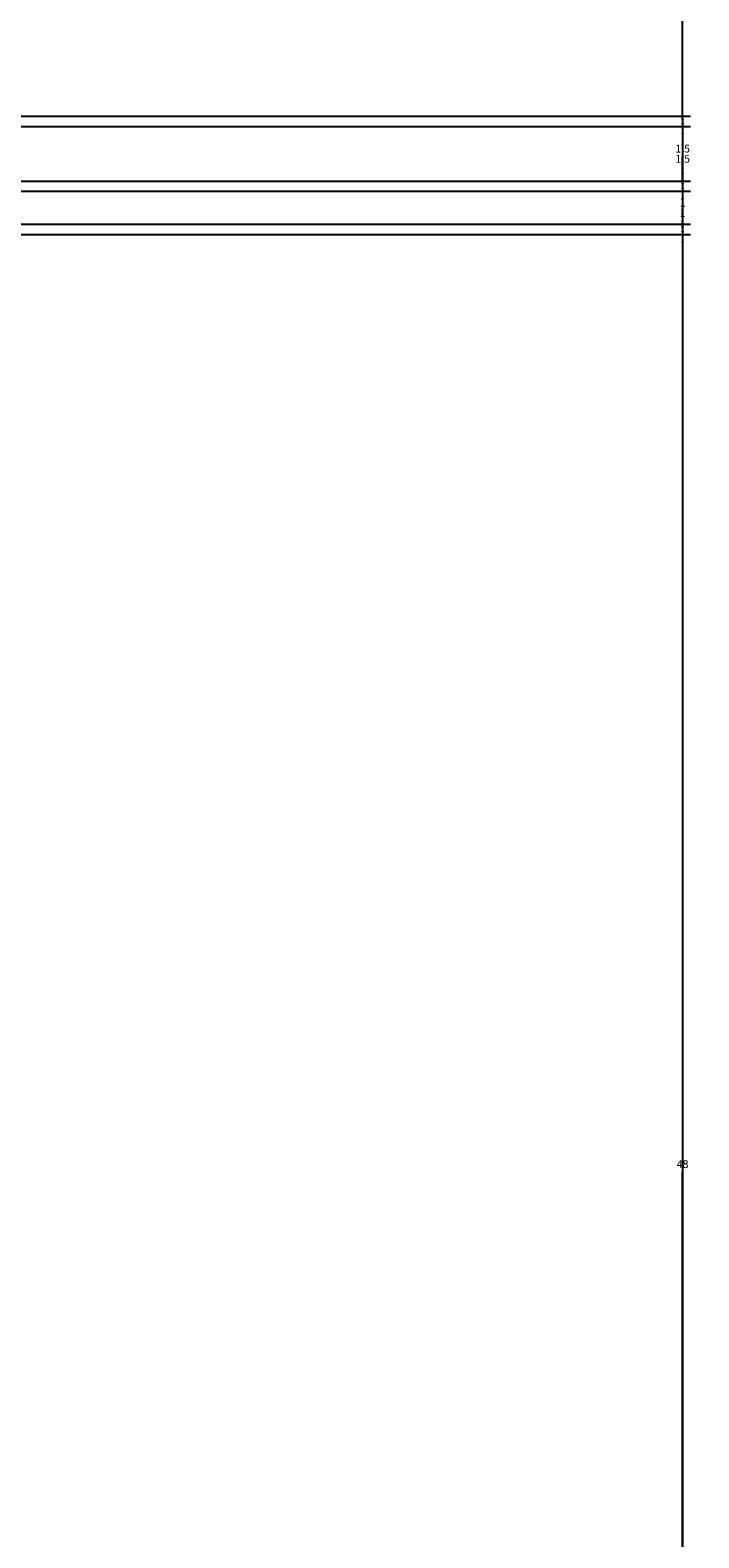
# Model space of a CAD drawing. Units: inches. Extents: x -6 to 289, y -8 to 323.
# Tile 76 of 107: x 273 to 289, y 194 to 229. Entities that reach past the tile are written whole.
import ezdxf

# ---------------------------------------------------------------- set-up
doc = ezdxf.new("R2010")
doc.units = ezdxf.units.IN
doc.header["$MEASUREMENT"] = 0
doc.layers.add('A-ANNO-DIMS', color=2, linetype='Continuous', lineweight=18)
doc.styles.get("Standard").update_dxf_attribs({"font": 'arial.ttf'})
doc.dimstyles.get("Standard").update_dxf_attribs({"dimtxt": 0.18, "dimasz": 0.18, "dimexe": 0.18, "dimexo": 0.0625, "dimgap": 0.09, "dimtad": 0, "dimtih": 1, "dimtoh": 1, "dimdec": 4, "dimzin": 0, "dimdsep": 46, "dimtxsty": 'Standard', "dimcen": 0.09, "dimadec": 0, "dimazin": 0, "dimtfac": 1, "dimtdec": 4, "dimtofl": 0, "dimtmove": 0, "dimatfit": 3, "dimfxl": 1, "dimtolj": 1, "dimtzin": 0, "dimarcsym": 0})

# ---------------------------------------------------------------- blocks, each defined once
blk = doc.blocks.new('*D25')
at = {"layer": 'A-ANNO-DIMS', "color": 0, "lineweight": -2, "transparency": 16777216}
for p, q in [((126.946, 226.654), (288.653, 226.654)), ((288.473, 226.474), (288.473, 202.836)), ((288.473, 178.834), (288.473, 202.472)), ((126.946, 178.654), (288.653, 178.654))]:
    blk.add_line(p, q, dxfattribs=at)
at = {"layer": 'A-ANNO-DIMS', "color": 0, "transparency": 16777216}
for points in [[(288.443, 226.474), (288.503, 226.474), (288.473, 226.654)], [(288.443, 178.834), (288.503, 178.834), (288.473, 178.654)]]:
    blk.add_solid(points, dxfattribs=at)
at = {"layer": 'Defpoints', "color": 0, "transparency": 16777216}
for p in [(126.883, 226.654), (288.473, 226.654), (126.883, 178.654)]:
    blk.add_point(p, dxfattribs=at)
at = {"layer": 'A-ANNO-DIMS', "color": 0, "transparency": 16777216, "insert": (288.473, 202.654), "char_height": 0.18, "attachment_point": 5}
blk.add_mtext('\\A1;48', dxfattribs=at)
blk = doc.blocks.new('*D26')
at = {"layer": 'A-ANNO-DIMS', "color": 0, "lineweight": -2, "transparency": 16777216}
for p, q in [((247.226, 247.289), (288.653, 247.289)), ((288.473, 247.109), (288.473, 237.153)), ((288.473, 226.834), (288.473, 236.789)), ((126.946, 226.654), (288.653, 226.654))]:
    blk.add_line(p, q, dxfattribs=at)
at = {"layer": 'A-ANNO-DIMS', "color": 0, "transparency": 16777216}
for points in [[(288.443, 247.109), (288.503, 247.109), (288.473, 247.289)], [(288.443, 226.834), (288.503, 226.834), (288.473, 226.654)]]:
    blk.add_solid(points, dxfattribs=at)
at = {"layer": 'Defpoints', "color": 0, "transparency": 16777216}
for p in [(247.164, 247.289), (288.473, 247.289), (126.883, 226.654)]:
    blk.add_point(p, dxfattribs=at)
at = {"layer": 'A-ANNO-DIMS', "color": 0, "transparency": 16777216, "insert": (288.473, 236.971), "char_height": 0.18, "attachment_point": 5}
blk.add_mtext('\\A1;20.635', dxfattribs=at)
blk = doc.blocks.new('*D37')
at = {"layer": 'A-ANNO-DIMS', "color": 0, "lineweight": -2, "transparency": 16777216}
for p, q in [((166.446, 224.154), (288.653, 224.154)), ((288.473, 223.974), (288.473, 202.836)), ((288.473, 181.334), (288.473, 202.472)), ((166.446, 181.154), (288.653, 181.154))]:
    blk.add_line(p, q, dxfattribs=at)
at = {"layer": 'A-ANNO-DIMS', "color": 0, "transparency": 16777216}
for points in [[(288.443, 223.974), (288.503, 223.974), (288.473, 224.154)], [(288.443, 181.334), (288.503, 181.334), (288.473, 181.154)]]:
    blk.add_solid(points, dxfattribs=at)
at = {"layer": 'Defpoints', "color": 0, "transparency": 16777216}
for p in [(166.383, 224.154), (288.473, 224.154), (166.383, 181.154)]:
    blk.add_point(p, dxfattribs=at)
at = {"layer": 'A-ANNO-DIMS', "color": 0, "transparency": 16777216, "insert": (288.473, 202.654), "char_height": 0.18, "attachment_point": 5}
blk.add_mtext('\\A1;43', dxfattribs=at)
blk = doc.blocks.new('*D38')
at = {"layer": 'A-ANNO-DIMS', "color": 0, "lineweight": -2, "transparency": 16777216}
for p, q in [((167.446, 225.154), (288.653, 225.154)), ((288.473, 224.974), (288.473, 224.834)), ((288.473, 224.334), (288.473, 224.474)), ((166.446, 224.154), (288.653, 224.154))]:
    blk.add_line(p, q, dxfattribs=at)
at = {"layer": 'A-ANNO-DIMS', "color": 0, "transparency": 16777216}
for points in [[(288.443, 224.974), (288.503, 224.974), (288.473, 225.154)], [(288.443, 224.334), (288.503, 224.334), (288.473, 224.154)]]:
    blk.add_solid(points, dxfattribs=at)
at = {"layer": 'Defpoints', "color": 0, "transparency": 16777216}
for p in [(167.383, 225.154), (288.473, 225.154), (166.383, 224.154)]:
    blk.add_point(p, dxfattribs=at)
at = {"layer": 'A-ANNO-DIMS', "color": 0, "transparency": 16777216, "insert": (288.473, 224.654), "char_height": 0.18, "attachment_point": 5}
blk.add_mtext('\\A1;1', dxfattribs=at)
blk = doc.blocks.new('*D39')
at = {"layer": 'A-ANNO-DIMS', "color": 0, "lineweight": -2, "transparency": 16777216}
for p, q in [((168.946, 226.654), (288.653, 226.654)), ((288.473, 226.474), (288.473, 226.086)), ((288.473, 225.334), (288.473, 225.722)), ((167.446, 225.154), (288.653, 225.154))]:
    blk.add_line(p, q, dxfattribs=at)
at = {"layer": 'A-ANNO-DIMS', "color": 0, "transparency": 16777216}
for points in [[(288.443, 226.474), (288.503, 226.474), (288.473, 226.654)], [(288.443, 225.334), (288.503, 225.334), (288.473, 225.154)]]:
    blk.add_solid(points, dxfattribs=at)
at = {"layer": 'Defpoints', "color": 0, "transparency": 16777216}
for p in [(168.883, 226.654), (288.473, 226.654), (167.383, 225.154)]:
    blk.add_point(p, dxfattribs=at)
at = {"layer": 'A-ANNO-DIMS', "color": 0, "transparency": 16777216, "insert": (288.473, 225.904), "char_height": 0.18, "attachment_point": 5}
blk.add_mtext('\\A1;1.5', dxfattribs=at)
blk = doc.blocks.new('*D47')
at = {"layer": 'A-ANNO-DIMS', "color": 0, "lineweight": -2, "transparency": 16777216}
for p, q in [((233.854, 224.389), (288.653, 224.389)), ((288.473, 224.209), (288.473, 193.55)), ((288.473, 162.528), (288.473, 193.187)), ((236.354, 162.348), (288.653, 162.348))]:
    blk.add_line(p, q, dxfattribs=at)
at = {"layer": 'A-ANNO-DIMS', "color": 0, "transparency": 16777216}
for points in [[(288.443, 224.209), (288.503, 224.209), (288.473, 224.389)], [(288.443, 162.528), (288.503, 162.528), (288.473, 162.348)]]:
    blk.add_solid(points, dxfattribs=at)
at = {"layer": 'Defpoints', "color": 0, "transparency": 16777216}
for p in [(233.792, 224.389), (288.473, 224.389), (236.292, 162.348)]:
    blk.add_point(p, dxfattribs=at)
at = {"layer": 'A-ANNO-DIMS', "color": 0, "transparency": 16777216, "insert": (288.473, 193.369), "char_height": 0.18, "attachment_point": 5}
blk.add_mtext('\\A1;62.04', dxfattribs=at)
blk = doc.blocks.new('*D48')
at = {"layer": 'A-ANNO-DIMS', "color": 0, "lineweight": -2, "transparency": 16777216}
for p, q in [((234.854, 225.389), (288.653, 225.389)), ((288.473, 225.209), (288.473, 225.069)), ((288.473, 224.569), (288.473, 224.708)), ((233.854, 224.389), (288.653, 224.389))]:
    blk.add_line(p, q, dxfattribs=at)
at = {"layer": 'A-ANNO-DIMS', "color": 0, "transparency": 16777216}
for points in [[(288.443, 225.209), (288.503, 225.209), (288.473, 225.389)], [(288.443, 224.569), (288.503, 224.569), (288.473, 224.389)]]:
    blk.add_solid(points, dxfattribs=at)
at = {"layer": 'Defpoints', "color": 0, "transparency": 16777216}
for p in [(234.792, 225.389), (288.473, 225.389), (233.792, 224.389)]:
    blk.add_point(p, dxfattribs=at)
at = {"layer": 'A-ANNO-DIMS', "color": 0, "transparency": 16777216, "insert": (288.473, 224.889), "char_height": 0.18, "attachment_point": 5}
blk.add_mtext('\\A1;1', dxfattribs=at)
blk = doc.blocks.new('*D49')
at = {"layer": 'A-ANNO-DIMS', "color": 0, "lineweight": -2, "transparency": 16777216}
for p, q in [((236.354, 226.889), (288.653, 226.889)), ((288.473, 226.709), (288.473, 226.321)), ((288.473, 225.569), (288.473, 225.957)), ((234.854, 225.389), (288.653, 225.389))]:
    blk.add_line(p, q, dxfattribs=at)
at = {"layer": 'A-ANNO-DIMS', "color": 0, "transparency": 16777216}
for points in [[(288.443, 226.709), (288.503, 226.709), (288.473, 226.889)], [(288.443, 225.569), (288.503, 225.569), (288.473, 225.389)]]:
    blk.add_solid(points, dxfattribs=at)
at = {"layer": 'Defpoints', "color": 0, "transparency": 16777216}
for p in [(236.292, 226.889), (288.473, 226.889), (234.792, 225.389)]:
    blk.add_point(p, dxfattribs=at)
at = {"layer": 'A-ANNO-DIMS', "color": 0, "transparency": 16777216, "insert": (288.473, 226.139), "char_height": 0.18, "attachment_point": 5}
blk.add_mtext('\\A1;1.5', dxfattribs=at)

msp = doc.modelspace()

# ---------------------------------------------------------------- dimensions: what is measured, and where the dimension line sits
at = {"layer": 'A-ANNO-DIMS'}
for base, p1, p2, override, picture, middle in [((288.4733, 247.2888), (126.8835, 226.654), (247.1638, 247.2888), {"dimdec": 3, "dimlfac": 1, "dimrnd": 0, "dimzin": 0, "dimdsep": 46, "dimlunit": 2}, '*D26', (288.4733, 236.9714)), ((288.4733, 226.654), (126.8835, 178.654), (126.8835, 226.654), {"dimdec": 0, "dimlfac": 1, "dimrnd": 0, "dimzin": 0, "dimdsep": 46, "dimlunit": 2}, '*D25', (288.4733, 202.654)), ((288.4733, 226.654), (167.3835, 225.154), (168.8835, 226.654), {"dimdec": 1, "dimlfac": 1, "dimrnd": 0, "dimzin": 0, "dimdsep": 46, "dimlunit": 2}, '*D39', (288.4733, 225.904)), ((288.4733, 226.8887), (234.7918, 225.3887), (236.2918, 226.8887), {"dimdec": 1, "dimlfac": 1, "dimrnd": 0, "dimzin": 0, "dimdsep": 46, "dimlunit": 2}, '*D49', (288.4733, 226.1387)), ((288.4733, 225.3887), (233.7918, 224.3887), (234.7918, 225.3887), {"dimdec": 0, "dimlfac": 1, "dimrnd": 0, "dimzin": 0, "dimdsep": 46, "dimlunit": 2}, '*D48', (288.4733, 224.8887)), ((288.4733, 225.154), (166.3835, 224.154), (167.3835, 225.154), {"dimdec": 0, "dimlfac": 1, "dimrnd": 0, "dimzin": 0, "dimdsep": 46, "dimlunit": 2}, '*D38', (288.4733, 224.654)), ((288.4733, 224.3887), (236.2918, 162.3484), (233.7918, 224.3887), {"dimdec": 2, "dimlfac": 1, "dimrnd": 0, "dimzin": 0, "dimdsep": 46, "dimlunit": 2}, '*D47', (288.4733, 193.3685)), ((288.4733, 224.154), (166.3835, 181.154), (166.3835, 224.154), {"dimdec": 0, "dimlfac": 1, "dimrnd": 0, "dimzin": 0, "dimdsep": 46, "dimlunit": 2}, '*D37', (288.4733, 202.654))]:
    dim = msp.add_linear_dim(base=base, p1=p1, p2=p2, angle=90, dimstyle='Standard', override=override, dxfattribs=at)
    dim.commit()
    dim.dimension.update_dxf_attribs({"geometry": picture, "text_midpoint": middle})

doc.saveas('drawing.dxf')
